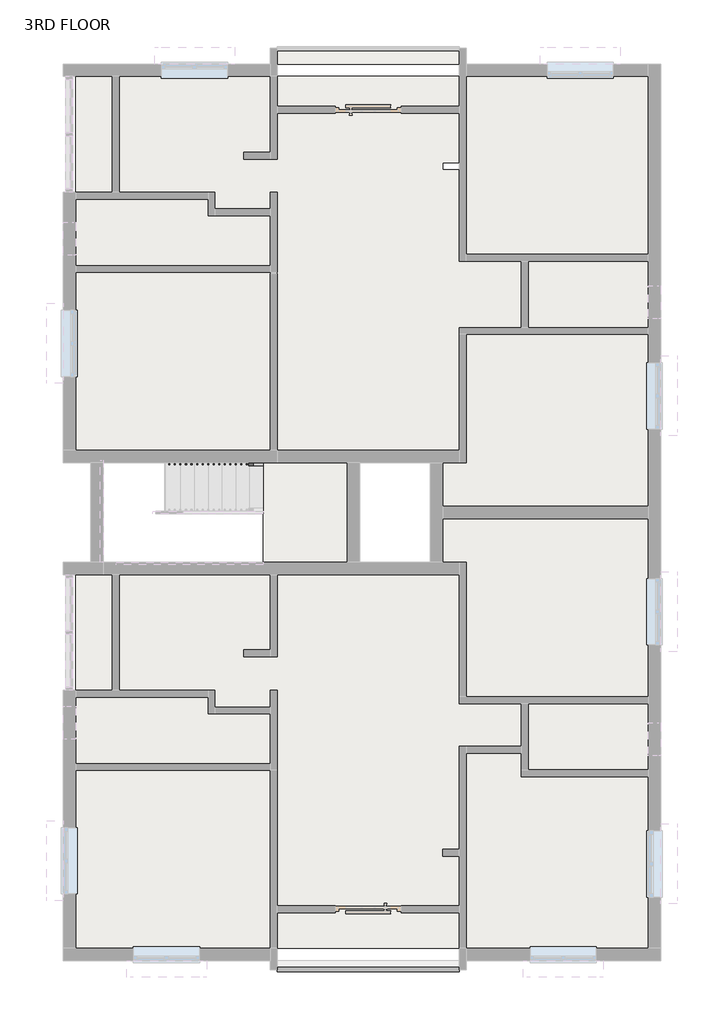
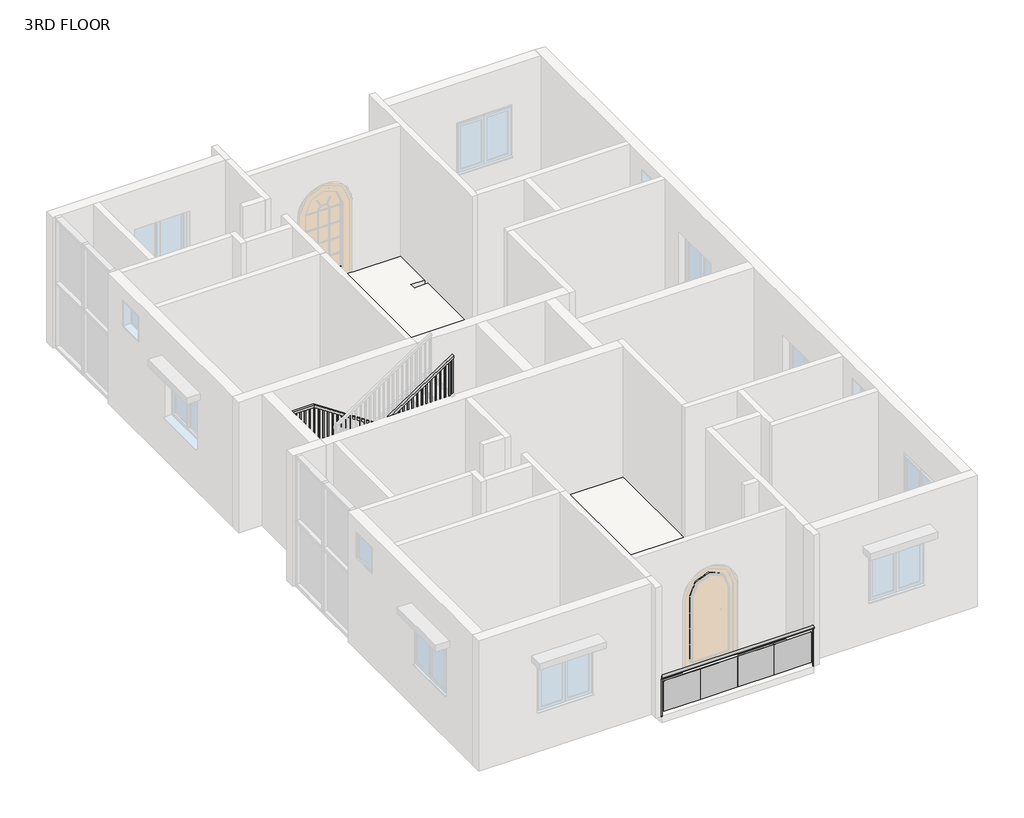
# One storey, part 3 of 4: 5 slabs, 2 railings.
"""IFC4 building model written with IfcOpenShell, lengths in millimetres."""

from ifc_helpers import new_model, si_unit, point, frame, origin, place, context, project, spatial, polyline, ellipse_curve, trimmed, outline, extrude, faceted_brep, element, save
from ifc_brep_helpers import plane_surface, extruded_surface, advanced_brep

model = new_model("IFC4")

# Units and contexts
model_context = context("Model", 3, world=origin())
ifc_project = project(units=[si_unit("LENGTHUNIT", "METRE", prefix="MILLI")], contexts=[model_context])

# Site, building, storey
site = spatial("IfcSite", under=ifc_project)
building = spatial("IfcBuilding", under=site)
storey = spatial("IfcBuildingStorey", under=building, Name="3RD FLOOR", Elevation=12192.0)

# Railings
placement = place(None, origin())
element("IfcRailing", 1, ObjectType="Glass Panel - Bottom Fill 2", at=placement, inside=storey, context=model_context, shape_type="SolidModel", body=[
    advanced_brep(
    [(-2494.0012202, -3358.1292559, 13106.4), (-2494.0012202, -3434.3292559, 13106.4), (858.7987798, -3358.1292559, 13106.4), (858.7987798, -3434.3292559, 13106.4)],
    [
        (0, 1, ellipse_curve(frame((-2494.0012202, -3396.2292559, 13106.4), z_axis=(-1.0, 0.0, 0.0), x_axis=(0.0, -1.0, 0.0)), 38.1, 28.575)),
        (1, 0, ellipse_curve(frame((-2494.0012202, -3396.2292559, 13106.4), z_axis=(-1.0, 0.0, 0.0), x_axis=(0.0, -1.0, 0.0)), 38.1, 28.575)),
        (2, 3, ellipse_curve(frame((858.7987798, -3396.2292559, 13106.4), z_axis=(1.0, 0.0, 0.0), x_axis=(0.0, -1.0, 0.0)), 38.1, 28.575)),
        (3, 2, ellipse_curve(frame((858.7987798, -3396.2292559, 13106.4), z_axis=(1.0, 0.0, 0.0), x_axis=(0.0, -1.0, 0.0)), 38.1, 28.575)),
        (0, 2),
        (3, 1),
    ],
    [
        plane_surface(frame((-2494.0012202, -3396.2292559, 13106.4), z_axis=(-1.0, 0.0, 0.0), x_axis=(0.0, 1.0, 0.0))),
        plane_surface(frame((858.7987798, -3396.2292559, 13106.4), z_axis=(1.0, 0.0, 0.0), x_axis=(0.0, 1.0, 0.0))),
        extruded_surface(trimmed(ellipse_curve(frame((858.7987798, -3396.2292559, 13106.4), z_axis=(-1.0, 0.0, 0.0), x_axis=(0.0, -1.0, 0.0)), 38.1, 28.575), [point((858.7987798, -3358.1292559, 13106.4))], [point((858.7987798, -3434.3292559, 13106.4))], True, "CARTESIAN"), (-3352.7999999999997, 0.0, 0.0), 3352.7999999999997),
        extruded_surface(trimmed(ellipse_curve(frame((858.7987798, -3396.2292559, 13106.4), z_axis=(-1.0, 0.0, 0.0), x_axis=(0.0, -1.0, 0.0)), 38.1, 28.575), [point((858.7987798, -3434.3292559, 13106.4))], [point((858.7987798, -3358.1292559, 13106.4))], True, "CARTESIAN"), (-3352.7999999999997, 0.0, 0.0), 3352.7999999999997),
    ],
    [
        (0, [[1, 2]]),
        (1, [[3, 4]]),
        (2, [[-1, 5, -4, 6]]),
        (3, [[-2, -6, -3, -5]]),
    ],
),
    extrude(outline(polyline([(-4.8012202, -3402.7644129), (-4.8012202, -3396.4144129), (807.9987798, -3396.4144129), (807.9987798, -3402.7644129), (-4.8012202, -3402.7644129)])), frame((0.0, 0.0, 12293.6), z_axis=(0.0, 0.0, 1.0), x_axis=(1.0, 0.0, 0.0)), (0.0, 0.0, 1.0), 711.2),
    extrude(outline(polyline([(-817.6012202, -3402.7644129), (-817.6012202, -3396.4144129), (-4.8012202, -3396.4144129), (-4.8012202, -3402.7644129), (-817.6012202, -3402.7644129)])), frame((0.0, 0.0, 12293.6), z_axis=(0.0, 0.0, 1.0), x_axis=(1.0, 0.0, 0.0)), (0.0, 0.0, 1.0), 711.2),
    extrude(outline(polyline([(-1630.4012202, -3402.7644129), (-1630.4012202, -3396.4144129), (-817.6012202, -3396.4144129), (-817.6012202, -3402.7644129), (-1630.4012202, -3402.7644129)])), frame((0.0, 0.0, 12293.6), z_axis=(0.0, 0.0, 1.0), x_axis=(1.0, 0.0, 0.0)), (0.0, 0.0, 1.0), 711.2),
    extrude(outline(polyline([(-2443.2012202, -3402.7644129), (-2443.2012202, -3396.4144129), (-1630.4012202, -3396.4144129), (-1630.4012202, -3402.7644129), (-2443.2012202, -3402.7644129)])), frame((0.0, 0.0, 12293.6), z_axis=(0.0, 0.0, 1.0), x_axis=(1.0, 0.0, 0.0)), (0.0, 0.0, 1.0), 711.2),
    extrude(outline(polyline([(846.0987798, -3386.7042559), (865.1487798, -3386.7042559), (865.1487798, -3405.7542559), (846.0987798, -3405.7542559), (846.0987798, -3386.7042559)])), frame((0.0, 0.0, 12192.0), z_axis=(0.0, 0.0, 1.0), x_axis=(1.0, 0.0, 0.0)), (0.0, 0.0, 1.0), 885.825),
    extrude(outline(polyline([(-2500.3512202, -3386.7042559), (-2481.3012202, -3386.7042559), (-2481.3012202, -3405.7542559), (-2500.3512202, -3405.7542559), (-2500.3512202, -3386.7042559)])), frame((0.0, 0.0, 12192.0), z_axis=(0.0, 0.0, 1.0), x_axis=(1.0, 0.0, 0.0)), (0.0, 0.0, 1.0), 885.825),
])
element("IfcRailing", 2, ObjectType="Handrail - Rectangular", at=placement, inside=storey, context=model_context, shape_type="SolidModel", body=[
    faceted_brep([(-2748.0012202, 5879.8309003, 13275.7333333), (-2748.0012202, 5879.8309003, 13214.6793317), (-2748.0012202, 5930.6309003, 13214.6793317), (-2748.0012202, 5930.6309003, 13275.7333333), (-4780.0012202, 5879.8309003, 14630.4), (-4795.3822226, 5879.8309003, 14579.6), (-4795.3822226, 5930.6309003, 14579.6), (-4780.0012202, 5930.6309003, 14630.4), (-5643.6012202, 5879.8309003, 14630.4), (-5643.6012202, 5879.8309003, 14579.6), (-5694.4012202, 5930.6309003, 14579.6), (-5694.4012202, 5930.6309003, 14630.4), (-5643.6012202, 4152.6309003, 14630.4), (-5643.6012202, 4152.6309003, 14579.6), (-5694.4012202, 4101.8309003, 14579.6), (-5694.4012202, 4101.8309003, 14630.4), (-5034.0012202, 4152.6309003, 14630.4), (-5018.6202178, 4152.6309003, 14579.6), (-5018.6202178, 4101.8309003, 14579.6), (-5034.0012202, 4101.8309003, 14630.4), (-2748.0012202, 4152.6309003, 16154.4), (-2748.0012202, 4101.8309003, 16154.4), (-2748.0012202, 4101.8309003, 16093.3459984), (-2748.0012202, 4152.6309003, 16093.3459984)], [[[0, 1, 2, 3]], [[1, 0, 4, 5]], [[2, 1, 5, 6]], [[3, 2, 6, 7]], [[0, 3, 7, 4]], [[5, 4, 8, 9]], [[6, 5, 9, 10]], [[7, 6, 10, 11]], [[4, 7, 11, 8]], [[9, 8, 12, 13]], [[10, 9, 13, 14]], [[11, 10, 14, 15]], [[8, 11, 15, 12]], [[13, 12, 16, 17]], [[14, 13, 17, 18]], [[15, 14, 18, 19]], [[12, 15, 19, 16]], [[20, 21, 22, 23]], [[17, 16, 20, 23]], [[18, 17, 23, 22]], [[19, 18, 22, 21]], [[16, 19, 21, 20]]]),
    extrude(outline(polyline([(16048.8959984, -2814.6762202), (16036.1959984, -2833.7262202), (15070.6666667, -2833.7262202), (15070.6666667, -2814.6762202), (16048.8959984, -2814.6762202)])), frame((0.0, 4117.7059003, 0.0), z_axis=(0.0, 1.0, 0.0), x_axis=(0.0, 0.0, 1.0)), (0.0, 0.0, 1.0), 19.05),
    extrude(outline(polyline([(15981.1626651, -2916.2762202), (15968.4626651, -2935.3262202), (15070.6666667, -2935.3262202), (15070.6666667, -2916.2762202), (15981.1626651, -2916.2762202)])), frame((0.0, 4117.7059003, 0.0), z_axis=(0.0, 1.0, 0.0), x_axis=(0.0, 0.0, 1.0)), (0.0, 0.0, 1.0), 19.05),
    extrude(outline(polyline([(15913.4293317, -3017.8762202), (15900.7293317, -3036.9262202), (14901.3333333, -3036.9262202), (14901.3333333, -3017.8762202), (15913.4293317, -3017.8762202)])), frame((0.0, 4117.7059003, 0.0), z_axis=(0.0, 1.0, 0.0), x_axis=(0.0, 0.0, 1.0)), (0.0, 0.0, 1.0), 19.05),
    extrude(outline(polyline([(15845.6959984, -3119.4762202), (15832.9959984, -3138.5262202), (14901.3333333, -3138.5262202), (14901.3333333, -3119.4762202), (15845.6959984, -3119.4762202)])), frame((0.0, 4117.7059003, 0.0), z_axis=(0.0, 1.0, 0.0), x_axis=(0.0, 0.0, 1.0)), (0.0, 0.0, 1.0), 19.05),
    extrude(outline(polyline([(15777.9626651, -3221.0762202), (15765.2626651, -3240.1262202), (14901.3333333, -3240.1262202), (14901.3333333, -3221.0762202), (15777.9626651, -3221.0762202)])), frame((0.0, 4117.7059003, 0.0), z_axis=(0.0, 1.0, 0.0), x_axis=(0.0, 0.0, 1.0)), (0.0, 0.0, 1.0), 19.05),
    extrude(outline(polyline([(15710.2293317, -3322.6762202), (15697.5293317, -3341.7262202), (14732.0, -3341.7262202), (14732.0, -3322.6762202), (15710.2293317, -3322.6762202)])), frame((0.0, 4117.7059003, 0.0), z_axis=(0.0, 1.0, 0.0), x_axis=(0.0, 0.0, 1.0)), (0.0, 0.0, 1.0), 19.05),
    extrude(outline(polyline([(15642.4959984, -3424.2762202), (15629.7959984, -3443.3262202), (14732.0, -3443.3262202), (14732.0, -3424.2762202), (15642.4959984, -3424.2762202)])), frame((0.0, 4117.7059003, 0.0), z_axis=(0.0, 1.0, 0.0), x_axis=(0.0, 0.0, 1.0)), (0.0, 0.0, 1.0), 19.05),
    extrude(outline(polyline([(15574.7626651, -3525.8762202), (15562.0626651, -3544.9262202), (14562.6666667, -3544.9262202), (14562.6666667, -3525.8762202), (15574.7626651, -3525.8762202)])), frame((0.0, 4117.7059003, 0.0), z_axis=(0.0, 1.0, 0.0), x_axis=(0.0, 0.0, 1.0)), (0.0, 0.0, 1.0), 19.05),
    extrude(outline(polyline([(15507.0293317, -3627.4762202), (15494.3293317, -3646.5262202), (14562.6666667, -3646.5262202), (14562.6666667, -3627.4762202), (15507.0293317, -3627.4762202)])), frame((0.0, 4117.7059003, 0.0), z_axis=(0.0, 1.0, 0.0), x_axis=(0.0, 0.0, 1.0)), (0.0, 0.0, 1.0), 19.05),
    extrude(outline(polyline([(15439.2959984, -3729.0762202), (15426.5959984, -3748.1262202), (14562.6666667, -3748.1262202), (14562.6666667, -3729.0762202), (15439.2959984, -3729.0762202)])), frame((0.0, 4117.7059003, 0.0), z_axis=(0.0, 1.0, 0.0), x_axis=(0.0, 0.0, 1.0)), (0.0, 0.0, 1.0), 19.05),
    extrude(outline(polyline([(15371.5626651, -3830.6762202), (15358.8626651, -3849.7262202), (14393.3333333, -3849.7262202), (14393.3333333, -3830.6762202), (15371.5626651, -3830.6762202)])), frame((0.0, 4117.7059003, 0.0), z_axis=(0.0, 1.0, 0.0), x_axis=(0.0, 0.0, 1.0)), (0.0, 0.0, 1.0), 19.05),
    extrude(outline(polyline([(15303.8293317, -3932.2762202), (15291.1293317, -3951.3262202), (14393.3333333, -3951.3262202), (14393.3333333, -3932.2762202), (15303.8293317, -3932.2762202)])), frame((0.0, 4117.7059003, 0.0), z_axis=(0.0, 1.0, 0.0), x_axis=(0.0, 0.0, 1.0)), (0.0, 0.0, 1.0), 19.05),
    extrude(outline(polyline([(15236.0959984, -4033.8762202), (15223.3959984, -4052.9262202), (14224.0, -4052.9262202), (14224.0, -4033.8762202), (15236.0959984, -4033.8762202)])), frame((0.0, 4117.7059003, 0.0), z_axis=(0.0, 1.0, 0.0), x_axis=(0.0, 0.0, 1.0)), (0.0, 0.0, 1.0), 19.05),
    extrude(outline(polyline([(15168.3626651, -4135.4762202), (15155.6626651, -4154.5262202), (14224.0, -4154.5262202), (14224.0, -4135.4762202), (15168.3626651, -4135.4762202)])), frame((0.0, 4117.7059003, 0.0), z_axis=(0.0, 1.0, 0.0), x_axis=(0.0, 0.0, 1.0)), (0.0, 0.0, 1.0), 19.05),
    extrude(outline(polyline([(15100.6293317, -4237.0762202), (15087.9293317, -4256.1262202), (14224.0, -4256.1262202), (14224.0, -4237.0762202), (15100.6293317, -4237.0762202)])), frame((0.0, 4117.7059003, 0.0), z_axis=(0.0, 1.0, 0.0), x_axis=(0.0, 0.0, 1.0)), (0.0, 0.0, 1.0), 19.05),
    extrude(outline(polyline([(15032.8959984, -4338.6762202), (15020.1959984, -4357.7262202), (14054.6666667, -4357.7262202), (14054.6666667, -4338.6762202), (15032.8959984, -4338.6762202)])), frame((0.0, 4117.7059003, 0.0), z_axis=(0.0, 1.0, 0.0), x_axis=(0.0, 0.0, 1.0)), (0.0, 0.0, 1.0), 19.05),
    extrude(outline(polyline([(14965.1626651, -4440.2762202), (14952.4626651, -4459.3262202), (14054.6666667, -4459.3262202), (14054.6666667, -4440.2762202), (14965.1626651, -4440.2762202)])), frame((0.0, 4117.7059003, 0.0), z_axis=(0.0, 1.0, 0.0), x_axis=(0.0, 0.0, 1.0)), (0.0, 0.0, 1.0), 19.05),
    extrude(outline(polyline([(14897.4293317, -4541.8762202), (14884.7293317, -4560.9262202), (13885.3333333, -4560.9262202), (13885.3333333, -4541.8762202), (14897.4293317, -4541.8762202)])), frame((0.0, 4117.7059003, 0.0), z_axis=(0.0, 1.0, 0.0), x_axis=(0.0, 0.0, 1.0)), (0.0, 0.0, 1.0), 19.05),
    extrude(outline(polyline([(14829.6959984, -4643.4762202), (14816.9959984, -4662.5262202), (13885.3333333, -4662.5262202), (13885.3333333, -4643.4762202), (14829.6959984, -4643.4762202)])), frame((0.0, 4117.7059003, 0.0), z_axis=(0.0, 1.0, 0.0), x_axis=(0.0, 0.0, 1.0)), (0.0, 0.0, 1.0), 19.05),
    extrude(outline(polyline([(14761.9626651, -4745.0762202), (14749.2626651, -4764.1262202), (13885.3333333, -4764.1262202), (13885.3333333, -4745.0762202), (14761.9626651, -4745.0762202)])), frame((0.0, 4117.7059003, 0.0), z_axis=(0.0, 1.0, 0.0), x_axis=(0.0, 0.0, 1.0)), (0.0, 0.0, 1.0), 19.05),
    extrude(outline(polyline([(14694.2293317, -4846.6762202), (14681.5293317, -4865.7262202), (13716.0, -4865.7262202), (13716.0, -4846.6762202), (14694.2293317, -4846.6762202)])), frame((0.0, 4117.7059003, 0.0), z_axis=(0.0, 1.0, 0.0), x_axis=(0.0, 0.0, 1.0)), (0.0, 0.0, 1.0), 19.05),
    extrude(outline(polyline([(14626.4959984, -4948.2762202), (14613.7959984, -4967.3262202), (13716.0, -4967.3262202), (13716.0, -4948.2762202), (14626.4959984, -4948.2762202)])), frame((0.0, 4117.7059003, 0.0), z_axis=(0.0, 1.0, 0.0), x_axis=(0.0, 0.0, 1.0)), (0.0, 0.0, 1.0), 19.05),
    extrude(outline(polyline([(-5068.9262202, 4117.7059003), (-5068.9262202, 4136.7559003), (-5049.8762202, 4136.7559003), (-5049.8762202, 4117.7059003), (-5068.9262202, 4117.7059003)])), frame((0.0, 0.0, 13716.0), z_axis=(0.0, 0.0, 1.0), x_axis=(1.0, 0.0, 0.0)), (0.0, 0.0, 1.0), 863.6),
    extrude(outline(polyline([(-5170.5262202, 4117.7059003), (-5170.5262202, 4136.7559003), (-5151.4762202, 4136.7559003), (-5151.4762202, 4117.7059003), (-5170.5262202, 4117.7059003)])), frame((0.0, 0.0, 13716.0), z_axis=(0.0, 0.0, 1.0), x_axis=(1.0, 0.0, 0.0)), (0.0, 0.0, 1.0), 863.6),
    extrude(outline(polyline([(-5272.1262202, 4117.7059003), (-5272.1262202, 4136.7559003), (-5253.0762202, 4136.7559003), (-5253.0762202, 4117.7059003), (-5272.1262202, 4117.7059003)])), frame((0.0, 0.0, 13716.0), z_axis=(0.0, 0.0, 1.0), x_axis=(1.0, 0.0, 0.0)), (0.0, 0.0, 1.0), 863.6),
    extrude(outline(polyline([(-5373.7262202, 4117.7059003), (-5373.7262202, 4136.7559003), (-5354.6762202, 4136.7559003), (-5354.6762202, 4117.7059003), (-5373.7262202, 4117.7059003)])), frame((0.0, 0.0, 13716.0), z_axis=(0.0, 0.0, 1.0), x_axis=(1.0, 0.0, 0.0)), (0.0, 0.0, 1.0), 863.6),
    extrude(outline(polyline([(-5475.3262202, 4117.7059003), (-5475.3262202, 4136.7559003), (-5456.2762202, 4136.7559003), (-5456.2762202, 4117.7059003), (-5475.3262202, 4117.7059003)])), frame((0.0, 0.0, 13716.0), z_axis=(0.0, 0.0, 1.0), x_axis=(1.0, 0.0, 0.0)), (0.0, 0.0, 1.0), 863.6),
    extrude(outline(polyline([(-5576.9262202, 4117.7059003), (-5576.9262202, 4136.7559003), (-5557.8762202, 4136.7559003), (-5557.8762202, 4117.7059003), (-5576.9262202, 4117.7059003)])), frame((0.0, 0.0, 13716.0), z_axis=(0.0, 0.0, 1.0), x_axis=(1.0, 0.0, 0.0)), (0.0, 0.0, 1.0), 863.6),
    extrude(outline(polyline([(-5678.5262202, 4187.5559003), (-5659.4762202, 4187.5559003), (-5659.4762202, 4168.5059003), (-5678.5262202, 4168.5059003), (-5678.5262202, 4187.5559003)])), frame((0.0, 0.0, 13716.0), z_axis=(0.0, 0.0, 1.0), x_axis=(1.0, 0.0, 0.0)), (0.0, 0.0, 1.0), 863.6),
    extrude(outline(polyline([(-5678.5262202, 4289.1559003), (-5659.4762202, 4289.1559003), (-5659.4762202, 4270.1059003), (-5678.5262202, 4270.1059003), (-5678.5262202, 4289.1559003)])), frame((0.0, 0.0, 13716.0), z_axis=(0.0, 0.0, 1.0), x_axis=(1.0, 0.0, 0.0)), (0.0, 0.0, 1.0), 863.6),
    extrude(outline(polyline([(-5678.5262202, 4390.7559003), (-5659.4762202, 4390.7559003), (-5659.4762202, 4371.7059003), (-5678.5262202, 4371.7059003), (-5678.5262202, 4390.7559003)])), frame((0.0, 0.0, 13716.0), z_axis=(0.0, 0.0, 1.0), x_axis=(1.0, 0.0, 0.0)), (0.0, 0.0, 1.0), 863.6),
    extrude(outline(polyline([(-5678.5262202, 4492.3559003), (-5659.4762202, 4492.3559003), (-5659.4762202, 4473.3059003), (-5678.5262202, 4473.3059003), (-5678.5262202, 4492.3559003)])), frame((0.0, 0.0, 13716.0), z_axis=(0.0, 0.0, 1.0), x_axis=(1.0, 0.0, 0.0)), (0.0, 0.0, 1.0), 863.6),
    extrude(outline(polyline([(-5678.5262202, 4593.9559003), (-5659.4762202, 4593.9559003), (-5659.4762202, 4574.9059003), (-5678.5262202, 4574.9059003), (-5678.5262202, 4593.9559003)])), frame((0.0, 0.0, 13716.0), z_axis=(0.0, 0.0, 1.0), x_axis=(1.0, 0.0, 0.0)), (0.0, 0.0, 1.0), 863.6),
    extrude(outline(polyline([(-5678.5262202, 4695.5559003), (-5659.4762202, 4695.5559003), (-5659.4762202, 4676.5059003), (-5678.5262202, 4676.5059003), (-5678.5262202, 4695.5559003)])), frame((0.0, 0.0, 13716.0), z_axis=(0.0, 0.0, 1.0), x_axis=(1.0, 0.0, 0.0)), (0.0, 0.0, 1.0), 863.6),
    extrude(outline(polyline([(-5678.5262202, 4797.1559003), (-5659.4762202, 4797.1559003), (-5659.4762202, 4778.1059003), (-5678.5262202, 4778.1059003), (-5678.5262202, 4797.1559003)])), frame((0.0, 0.0, 13716.0), z_axis=(0.0, 0.0, 1.0), x_axis=(1.0, 0.0, 0.0)), (0.0, 0.0, 1.0), 863.6),
    extrude(outline(polyline([(-5678.5262202, 4898.7559003), (-5659.4762202, 4898.7559003), (-5659.4762202, 4879.7059003), (-5678.5262202, 4879.7059003), (-5678.5262202, 4898.7559003)])), frame((0.0, 0.0, 13716.0), z_axis=(0.0, 0.0, 1.0), x_axis=(1.0, 0.0, 0.0)), (0.0, 0.0, 1.0), 863.6),
    extrude(outline(polyline([(-5678.5262202, 5000.3559003), (-5659.4762202, 5000.3559003), (-5659.4762202, 4981.3059003), (-5678.5262202, 4981.3059003), (-5678.5262202, 5000.3559003)])), frame((0.0, 0.0, 13716.0), z_axis=(0.0, 0.0, 1.0), x_axis=(1.0, 0.0, 0.0)), (0.0, 0.0, 1.0), 863.6),
    extrude(outline(polyline([(-5678.5262202, 5101.9559003), (-5659.4762202, 5101.9559003), (-5659.4762202, 5082.9059003), (-5678.5262202, 5082.9059003), (-5678.5262202, 5101.9559003)])), frame((0.0, 0.0, 13716.0), z_axis=(0.0, 0.0, 1.0), x_axis=(1.0, 0.0, 0.0)), (0.0, 0.0, 1.0), 863.6),
    extrude(outline(polyline([(-5678.5262202, 5203.5559003), (-5659.4762202, 5203.5559003), (-5659.4762202, 5184.5059003), (-5678.5262202, 5184.5059003), (-5678.5262202, 5203.5559003)])), frame((0.0, 0.0, 13716.0), z_axis=(0.0, 0.0, 1.0), x_axis=(1.0, 0.0, 0.0)), (0.0, 0.0, 1.0), 863.6),
    extrude(outline(polyline([(-5678.5262202, 5305.1559003), (-5659.4762202, 5305.1559003), (-5659.4762202, 5286.1059003), (-5678.5262202, 5286.1059003), (-5678.5262202, 5305.1559003)])), frame((0.0, 0.0, 13716.0), z_axis=(0.0, 0.0, 1.0), x_axis=(1.0, 0.0, 0.0)), (0.0, 0.0, 1.0), 863.6),
    extrude(outline(polyline([(-5678.5262202, 5406.7559003), (-5659.4762202, 5406.7559003), (-5659.4762202, 5387.7059003), (-5678.5262202, 5387.7059003), (-5678.5262202, 5406.7559003)])), frame((0.0, 0.0, 13716.0), z_axis=(0.0, 0.0, 1.0), x_axis=(1.0, 0.0, 0.0)), (0.0, 0.0, 1.0), 863.6),
    extrude(outline(polyline([(-5678.5262202, 5508.3559003), (-5659.4762202, 5508.3559003), (-5659.4762202, 5489.3059003), (-5678.5262202, 5489.3059003), (-5678.5262202, 5508.3559003)])), frame((0.0, 0.0, 13716.0), z_axis=(0.0, 0.0, 1.0), x_axis=(1.0, 0.0, 0.0)), (0.0, 0.0, 1.0), 863.6),
    extrude(outline(polyline([(-5678.5262202, 5609.9559003), (-5659.4762202, 5609.9559003), (-5659.4762202, 5590.9059003), (-5678.5262202, 5590.9059003), (-5678.5262202, 5609.9559003)])), frame((0.0, 0.0, 13716.0), z_axis=(0.0, 0.0, 1.0), x_axis=(1.0, 0.0, 0.0)), (0.0, 0.0, 1.0), 863.6),
    extrude(outline(polyline([(-5678.5262202, 5711.5559003), (-5659.4762202, 5711.5559003), (-5659.4762202, 5692.5059003), (-5678.5262202, 5692.5059003), (-5678.5262202, 5711.5559003)])), frame((0.0, 0.0, 13716.0), z_axis=(0.0, 0.0, 1.0), x_axis=(1.0, 0.0, 0.0)), (0.0, 0.0, 1.0), 863.6),
    extrude(outline(polyline([(-5678.5262202, 5813.1559003), (-5659.4762202, 5813.1559003), (-5659.4762202, 5794.1059003), (-5678.5262202, 5794.1059003), (-5678.5262202, 5813.1559003)])), frame((0.0, 0.0, 13716.0), z_axis=(0.0, 0.0, 1.0), x_axis=(1.0, 0.0, 0.0)), (0.0, 0.0, 1.0), 863.6),
    extrude(outline(polyline([(-5583.2762202, 5914.7559003), (-5583.2762202, 5895.7059003), (-5602.3262202, 5895.7059003), (-5602.3262202, 5914.7559003), (-5583.2762202, 5914.7559003)])), frame((0.0, 0.0, 13716.0), z_axis=(0.0, 0.0, 1.0), x_axis=(1.0, 0.0, 0.0)), (0.0, 0.0, 1.0), 863.6),
    extrude(outline(polyline([(-5481.6762202, 5914.7559003), (-5481.6762202, 5895.7059003), (-5500.7262202, 5895.7059003), (-5500.7262202, 5914.7559003), (-5481.6762202, 5914.7559003)])), frame((0.0, 0.0, 13716.0), z_axis=(0.0, 0.0, 1.0), x_axis=(1.0, 0.0, 0.0)), (0.0, 0.0, 1.0), 863.6),
    extrude(outline(polyline([(-5380.0762202, 5914.7559003), (-5380.0762202, 5895.7059003), (-5399.1262202, 5895.7059003), (-5399.1262202, 5914.7559003), (-5380.0762202, 5914.7559003)])), frame((0.0, 0.0, 13716.0), z_axis=(0.0, 0.0, 1.0), x_axis=(1.0, 0.0, 0.0)), (0.0, 0.0, 1.0), 863.6),
    extrude(outline(polyline([(-5278.4762202, 5914.7559003), (-5278.4762202, 5895.7059003), (-5297.5262202, 5895.7059003), (-5297.5262202, 5914.7559003), (-5278.4762202, 5914.7559003)])), frame((0.0, 0.0, 13716.0), z_axis=(0.0, 0.0, 1.0), x_axis=(1.0, 0.0, 0.0)), (0.0, 0.0, 1.0), 863.6),
    extrude(outline(polyline([(-5176.8762202, 5914.7559003), (-5176.8762202, 5895.7059003), (-5195.9262202, 5895.7059003), (-5195.9262202, 5914.7559003), (-5176.8762202, 5914.7559003)])), frame((0.0, 0.0, 13716.0), z_axis=(0.0, 0.0, 1.0), x_axis=(1.0, 0.0, 0.0)), (0.0, 0.0, 1.0), 863.6),
    extrude(outline(polyline([(-5075.2762202, 5914.7559003), (-5075.2762202, 5895.7059003), (-5094.3262202, 5895.7059003), (-5094.3262202, 5914.7559003), (-5075.2762202, 5914.7559003)])), frame((0.0, 0.0, 13716.0), z_axis=(0.0, 0.0, 1.0), x_axis=(1.0, 0.0, 0.0)), (0.0, 0.0, 1.0), 863.6),
    extrude(outline(polyline([(-4973.6762202, 5914.7559003), (-4973.6762202, 5895.7059003), (-4992.7262202, 5895.7059003), (-4992.7262202, 5914.7559003), (-4973.6762202, 5914.7559003)])), frame((0.0, 0.0, 13716.0), z_axis=(0.0, 0.0, 1.0), x_axis=(1.0, 0.0, 0.0)), (0.0, 0.0, 1.0), 863.6),
    extrude(outline(polyline([(-4872.0762202, 5914.7559003), (-4872.0762202, 5895.7059003), (-4891.1262202, 5895.7059003), (-4891.1262202, 5914.7559003), (-4872.0762202, 5914.7559003)])), frame((0.0, 0.0, 13716.0), z_axis=(0.0, 0.0, 1.0), x_axis=(1.0, 0.0, 0.0)), (0.0, 0.0, 1.0), 863.6),
    extrude(outline(polyline([(14562.9959984, -4770.4762202), (14575.6959984, -4789.5262202), (13716.0, -4789.5262202), (13716.0, -4770.4762202), (14562.9959984, -4770.4762202)])), frame((0.0, 5895.7059003, 0.0), z_axis=(0.0, 1.0, 0.0), x_axis=(0.0, 0.0, 1.0)), (0.0, 0.0, 1.0), 19.05),
    extrude(outline(polyline([(14495.2626651, -4668.8762202), (14507.9626651, -4687.9262202), (13546.6666667, -4687.9262202), (13546.6666667, -4668.8762202), (14495.2626651, -4668.8762202)])), frame((0.0, 5895.7059003, 0.0), z_axis=(0.0, 1.0, 0.0), x_axis=(0.0, 0.0, 1.0)), (0.0, 0.0, 1.0), 19.05),
    extrude(outline(polyline([(14427.5293317, -4567.2762202), (14440.2293317, -4586.3262202), (13546.6666667, -4586.3262202), (13546.6666667, -4567.2762202), (14427.5293317, -4567.2762202)])), frame((0.0, 5895.7059003, 0.0), z_axis=(0.0, 1.0, 0.0), x_axis=(0.0, 0.0, 1.0)), (0.0, 0.0, 1.0), 19.05),
    extrude(outline(polyline([(14359.7959984, -4465.6762202), (14372.4959984, -4484.7262202), (13377.3333333, -4484.7262202), (13377.3333333, -4465.6762202), (14359.7959984, -4465.6762202)])), frame((0.0, 5895.7059003, 0.0), z_axis=(0.0, 1.0, 0.0), x_axis=(0.0, 0.0, 1.0)), (0.0, 0.0, 1.0), 19.05),
    extrude(outline(polyline([(14292.0626651, -4364.0762202), (14304.7626651, -4383.1262202), (13377.3333333, -4383.1262202), (13377.3333333, -4364.0762202), (14292.0626651, -4364.0762202)])), frame((0.0, 5895.7059003, 0.0), z_axis=(0.0, 1.0, 0.0), x_axis=(0.0, 0.0, 1.0)), (0.0, 0.0, 1.0), 19.05),
    extrude(outline(polyline([(14224.3293317, -4262.4762202), (14237.0293317, -4281.5262202), (13377.3333333, -4281.5262202), (13377.3333333, -4262.4762202), (14224.3293317, -4262.4762202)])), frame((0.0, 5895.7059003, 0.0), z_axis=(0.0, 1.0, 0.0), x_axis=(0.0, 0.0, 1.0)), (0.0, 0.0, 1.0), 19.05),
    extrude(outline(polyline([(14156.5959984, -4160.8762202), (14169.2959984, -4179.9262202), (13208.0, -4179.9262202), (13208.0, -4160.8762202), (14156.5959984, -4160.8762202)])), frame((0.0, 5895.7059003, 0.0), z_axis=(0.0, 1.0, 0.0), x_axis=(0.0, 0.0, 1.0)), (0.0, 0.0, 1.0), 19.05),
    extrude(outline(polyline([(14088.8626651, -4059.2762202), (14101.5626651, -4078.3262202), (13208.0, -4078.3262202), (13208.0, -4059.2762202), (14088.8626651, -4059.2762202)])), frame((0.0, 5895.7059003, 0.0), z_axis=(0.0, 1.0, 0.0), x_axis=(0.0, 0.0, 1.0)), (0.0, 0.0, 1.0), 19.05),
    extrude(outline(polyline([(14021.1293317, -3957.6762202), (14033.8293317, -3976.7262202), (13038.6666667, -3976.7262202), (13038.6666667, -3957.6762202), (14021.1293317, -3957.6762202)])), frame((0.0, 5895.7059003, 0.0), z_axis=(0.0, 1.0, 0.0), x_axis=(0.0, 0.0, 1.0)), (0.0, 0.0, 1.0), 19.05),
    extrude(outline(polyline([(13953.3959984, -3856.0762202), (13966.0959984, -3875.1262202), (13038.6666667, -3875.1262202), (13038.6666667, -3856.0762202), (13953.3959984, -3856.0762202)])), frame((0.0, 5895.7059003, 0.0), z_axis=(0.0, 1.0, 0.0), x_axis=(0.0, 0.0, 1.0)), (0.0, 0.0, 1.0), 19.05),
    extrude(outline(polyline([(13885.6626651, -3754.4762202), (13898.3626651, -3773.5262202), (13038.6666667, -3773.5262202), (13038.6666667, -3754.4762202), (13885.6626651, -3754.4762202)])), frame((0.0, 5895.7059003, 0.0), z_axis=(0.0, 1.0, 0.0), x_axis=(0.0, 0.0, 1.0)), (0.0, 0.0, 1.0), 19.05),
    extrude(outline(polyline([(13817.9293317, -3652.8762202), (13830.6293317, -3671.9262202), (12869.3333333, -3671.9262202), (12869.3333333, -3652.8762202), (13817.9293317, -3652.8762202)])), frame((0.0, 5895.7059003, 0.0), z_axis=(0.0, 1.0, 0.0), x_axis=(0.0, 0.0, 1.0)), (0.0, 0.0, 1.0), 19.05),
    extrude(outline(polyline([(13750.1959984, -3551.2762202), (13762.8959984, -3570.3262202), (12869.3333333, -3570.3262202), (12869.3333333, -3551.2762202), (13750.1959984, -3551.2762202)])), frame((0.0, 5895.7059003, 0.0), z_axis=(0.0, 1.0, 0.0), x_axis=(0.0, 0.0, 1.0)), (0.0, 0.0, 1.0), 19.05),
    extrude(outline(polyline([(13682.4626651, -3449.6762202), (13695.1626651, -3468.7262202), (12700.0, -3468.7262202), (12700.0, -3449.6762202), (13682.4626651, -3449.6762202)])), frame((0.0, 5895.7059003, 0.0), z_axis=(0.0, 1.0, 0.0), x_axis=(0.0, 0.0, 1.0)), (0.0, 0.0, 1.0), 19.05),
    extrude(outline(polyline([(13614.7293317, -3348.0762202), (13627.4293317, -3367.1262202), (12700.0, -3367.1262202), (12700.0, -3348.0762202), (13614.7293317, -3348.0762202)])), frame((0.0, 5895.7059003, 0.0), z_axis=(0.0, 1.0, 0.0), x_axis=(0.0, 0.0, 1.0)), (0.0, 0.0, 1.0), 19.05),
    extrude(outline(polyline([(13546.9959984, -3246.4762202), (13559.6959984, -3265.5262202), (12700.0, -3265.5262202), (12700.0, -3246.4762202), (13546.9959984, -3246.4762202)])), frame((0.0, 5895.7059003, 0.0), z_axis=(0.0, 1.0, 0.0), x_axis=(0.0, 0.0, 1.0)), (0.0, 0.0, 1.0), 19.05),
    extrude(outline(polyline([(13479.2626651, -3144.8762202), (13491.9626651, -3163.9262202), (12530.6666667, -3163.9262202), (12530.6666667, -3144.8762202), (13479.2626651, -3144.8762202)])), frame((0.0, 5895.7059003, 0.0), z_axis=(0.0, 1.0, 0.0), x_axis=(0.0, 0.0, 1.0)), (0.0, 0.0, 1.0), 19.05),
    extrude(outline(polyline([(13411.5293317, -3043.2762202), (13424.2293317, -3062.3262202), (12530.6666667, -3062.3262202), (12530.6666667, -3043.2762202), (13411.5293317, -3043.2762202)])), frame((0.0, 5895.7059003, 0.0), z_axis=(0.0, 1.0, 0.0), x_axis=(0.0, 0.0, 1.0)), (0.0, 0.0, 1.0), 19.05),
    extrude(outline(polyline([(13343.7959984, -2941.6762202), (13356.4959984, -2960.7262202), (12361.3333333, -2960.7262202), (12361.3333333, -2941.6762202), (13343.7959984, -2941.6762202)])), frame((0.0, 5895.7059003, 0.0), z_axis=(0.0, 1.0, 0.0), x_axis=(0.0, 0.0, 1.0)), (0.0, 0.0, 1.0), 19.05),
    extrude(outline(polyline([(13276.0626651, -2840.0762202), (13288.7626651, -2859.1262202), (12361.3333333, -2859.1262202), (12361.3333333, -2840.0762202), (13276.0626651, -2840.0762202)])), frame((0.0, 5895.7059003, 0.0), z_axis=(0.0, 1.0, 0.0), x_axis=(0.0, 0.0, 1.0)), (0.0, 0.0, 1.0), 19.05),
    extrude(outline(polyline([(-5678.5262202, 4136.7559003), (-5659.4762202, 4136.7559003), (-5659.4762202, 4117.7059003), (-5678.5262202, 4117.7059003), (-5678.5262202, 4136.7559003)])), frame((0.0, 0.0, 13716.0), z_axis=(0.0, 0.0, 1.0), x_axis=(1.0, 0.0, 0.0)), (0.0, 0.0, 1.0), 863.6),
    extrude(outline(polyline([(-5659.4762202, 5914.7559003), (-5659.4762202, 5895.7059003), (-5678.5262202, 5895.7059003), (-5678.5262202, 5914.7559003), (-5659.4762202, 5914.7559003)])), frame((0.0, 0.0, 13716.0), z_axis=(0.0, 0.0, 1.0), x_axis=(1.0, 0.0, 0.0)), (0.0, 0.0, 1.0), 863.6),
    extrude(outline(polyline([(16093.3459984, -2748.0012202), (16080.6459984, -2767.0512202), (15070.6666667, -2767.0512202), (15070.6666667, -2748.0012202), (16093.3459984, -2748.0012202)])), frame((0.0, 4117.7059003, 0.0), z_axis=(0.0, 1.0, 0.0), x_axis=(0.0, 0.0, 1.0)), (0.0, 0.0, 1.0), 19.05),
    extrude(outline(polyline([(13214.6793317, -2748.0012202), (13227.3793317, -2767.0512202), (12361.3333333, -2767.0512202), (12361.3333333, -2748.0012202), (13214.6793317, -2748.0012202)])), frame((0.0, 5895.7059003, 0.0), z_axis=(0.0, 1.0, 0.0), x_axis=(0.0, 0.0, 1.0)), (0.0, 0.0, 1.0), 19.05),
])

# Slabs
element("IfcSlab", 3, ObjectType="FLOORING 6\"", at=placement, inside=storey, context=model_context, shape_type="SweptSolid", body=[
    extrude(outline(polyline([(-2621.0012202, 11645.6309003), (-3103.6012202, 11645.6309003), (-3103.6012202, 11518.6309003), (-2557.5012202, 11518.6309003), (-2494.0012202, 11518.6309003), (-2494.0012202, 13042.6309003), (858.7987798, 13042.6309003), (858.7987798, 11455.1309003), (553.9987798, 11455.1309003), (553.9987798, 11328.1309003), (858.7987798, 11328.1309003), (858.7987798, 9639.0309003), (2001.7987798, 9639.0309003), (2001.7987798, 8419.8309003), (858.7987798, 8419.8309003), (858.7987798, 6159.2309003), (-2494.0012202, 6159.2309003), (-2494.0012202, 9435.8309003), (-2494.0012202, 10909.0309003), (-2621.0012202, 10909.0309003), (-2621.0012202, 10604.2309003), (-3637.0012202, 10604.2309003), (-3637.0012202, 10909.0309003), (-6202.4012202, 10909.0309003), (-6202.4012202, 13042.6309003), (-2621.0012202, 13042.6309003), (-2621.0012202, 11645.6309003)])), frame((0.0, 0.0, 12039.6), z_axis=(0.0, 0.0, 1.0), x_axis=(1.0, 0.0, 0.0)), (0.0, 0.0, 1.0), 152.4),
])
element("IfcSlab", 4, ObjectType="FLOORING 6\"", at=placement, inside=storey, context=model_context, shape_type="SweptSolid", body=[
    extrude(outline(polyline([(4338.5987798, 13042.6309003), (4338.5987798, 9766.0309003), (985.7987798, 9766.0309003), (985.7987798, 13042.6309003), (4338.5987798, 13042.6309003)])), frame((0.0, 0.0, 12039.6), z_axis=(0.0, 0.0, 1.0), x_axis=(1.0, 0.0, 0.0)), (0.0, 0.0, 1.0), 152.4),
    extrude(outline(polyline([(4338.5987798, 9639.0309003), (4338.5987798, 8419.8309003), (2128.7987798, 8419.8309003), (2128.7987798, 9639.0309003), (4338.5987798, 9639.0309003)])), frame((0.0, 0.0, 12039.6), z_axis=(0.0, 0.0, 1.0), x_axis=(1.0, 0.0, 0.0)), (0.0, 0.0, 1.0), 152.4),
    extrude(outline(polyline([(-2621.0012202, 9435.8309003), (-2621.0012202, 6159.2309003), (-6202.4012202, 6159.2309003), (-6202.4012202, 9435.8309003), (-2621.0012202, 9435.8309003)])), frame((0.0, 0.0, 12039.6), z_axis=(0.0, 0.0, 1.0), x_axis=(1.0, 0.0, 0.0)), (0.0, 0.0, 1.0), 152.4),
    extrude(outline(polyline([(-2621.0012202, 9562.8309003), (-6202.4012202, 9562.8309003), (-6202.4012202, 10782.0309003), (-3764.0012202, 10782.0309003), (-3764.0012202, 10477.2309003), (-2621.0012202, 10477.2309003), (-2621.0012202, 9562.8309003)])), frame((0.0, 0.0, 12039.6), z_axis=(0.0, 0.0, 1.0), x_axis=(1.0, 0.0, 0.0)), (0.0, 0.0, 1.0), 152.4),
    extrude(outline(polyline([(553.9987798, 5930.6309003), (985.7987798, 5930.6309003), (985.7987798, 8292.8309003), (4338.5987798, 8292.8309003), (4338.5987798, 5130.5309003), (553.9987798, 5130.5309003), (553.9987798, 5930.6309003)])), frame((0.0, 0.0, 12039.6), z_axis=(0.0, 0.0, 1.0), x_axis=(1.0, 0.0, 0.0)), (0.0, 0.0, 1.0), 152.4),
])
element("IfcSlab", 5, ObjectType="FLOORING 6\"", at=placement, inside=storey, context=model_context, shape_type="SweptSolid", body=[
    extrude(outline(polyline([(985.7987798, 583.9309003), (2001.7987798, 583.9309003), (2001.7987798, 152.1309003), (4338.5987798, 152.1309003), (4338.5987798, -3010.1690997), (985.7987798, -3010.1690997), (985.7987798, 583.9309003)])), frame((0.0, 0.0, 12039.6), z_axis=(0.0, 0.0, 1.0), x_axis=(1.0, 0.0, 0.0)), (0.0, 0.0, 1.0), 152.4),
    extrude(outline(polyline([(-6203.9887202, -3010.1690997), (-6203.9887202, 266.4309003), (-2621.0012202, 266.4309003), (-2621.0012202, -3010.1690997), (-6203.9887202, -3010.1690997)])), frame((0.0, 0.0, 12039.6), z_axis=(0.0, 0.0, 1.0), x_axis=(1.0, 0.0, 0.0)), (0.0, 0.0, 1.0), 152.4),
    extrude(outline(polyline([(-2621.0012202, 393.4309003), (-6203.9887202, 393.4309003), (-6203.9887202, 1612.6309003), (-3764.0012202, 1612.6309003), (-3764.0012202, 1307.8309003), (-2621.0012202, 1307.8309003), (-2621.0012202, 393.4309003)])), frame((0.0, 0.0, 12039.6), z_axis=(0.0, 0.0, 1.0), x_axis=(1.0, 0.0, 0.0)), (0.0, 0.0, 1.0), 152.4),
    extrude(outline(polyline([(858.7987798, -3010.1690997), (-2494.0012202, -3010.1690997), (-2494.0012202, 1739.6309003), (-2621.0012202, 1739.6309003), (-2621.0012202, 1434.8309003), (-3637.0012202, 1434.8309003), (-3637.0012202, 1739.6309003), (-6203.9887202, 1739.6309003), (-6203.9887202, 3873.2309003), (-2621.0012202, 3873.2309003), (-2621.0012202, 2488.9309003), (-3103.6012202, 2488.9309003), (-3103.6012202, 2361.9309003), (-2494.0012202, 2361.9309003), (-2494.0012202, 3873.2309003), (858.7987798, 3873.2309003), (858.7987798, 1498.3309003), (2001.7987798, 1498.3309003), (2001.7987798, 710.9309003), (858.7987798, 710.9309003), (858.7987798, -3010.1690997)])), frame((0.0, 0.0, 12039.6), z_axis=(0.0, 0.0, 1.0), x_axis=(1.0, 0.0, 0.0)), (0.0, 0.0, 1.0), 152.4),
    extrude(outline(polyline([(985.7987798, 1625.3309003), (985.7987798, 4101.8309003), (553.9987798, 4101.8309003), (553.9987798, 4901.9309003), (4338.5987798, 4901.9309003), (4338.5987798, 1625.3309003), (985.7987798, 1625.3309003)])), frame((0.0, 0.0, 12039.6), z_axis=(0.0, 0.0, 1.0), x_axis=(1.0, 0.0, 0.0)), (0.0, 0.0, 1.0), 152.4),
    extrude(outline(polyline([(-2748.0012202, 4000.2309003), (-2748.0012202, 5981.4309003), (-2748.0012202, 6032.2309003), (-2494.0012202, 6032.2309003), (-2494.0012202, 5930.6309003), (-1198.6012202, 5930.6309003), (-1198.6012202, 4101.8309003), (-2494.0012202, 4101.8309003), (-2494.0012202, 4000.2309003), (-2748.0012202, 4000.2309003)])), frame((0.0, 0.0, 12039.6), z_axis=(0.0, 0.0, 1.0), x_axis=(1.0, 0.0, 0.0)), (0.0, 0.0, 1.0), 152.4),
])
element("IfcSlab", 6, ObjectType="bathroom tiles", at=placement, inside=storey, context=model_context, shape_type="SweptSolid", body=[
    extrude(outline(polyline([(858.7987798, 13563.3309003), (858.7987798, 13271.2309003), (-2494.0012202, 13271.2309003), (-2494.0012202, 13563.3309003), (858.7987798, 13563.3309003)])), frame((0.0, 0.0, 12039.6), z_axis=(0.0, 0.0, 1.0), x_axis=(1.0, 0.0, 0.0)), (0.0, 0.0, 1.0), 152.4),
])
element("IfcSlab", 7, ObjectType="bathroom tiles", at=placement, inside=storey, context=model_context, shape_type="SweptSolid", body=[
    extrude(outline(polyline([(4338.5987798, 1498.3309003), (4338.5987798, 279.1309003), (2128.7987798, 279.1309003), (2128.7987798, 1498.3309003), (4338.5987798, 1498.3309003)])), frame((0.0, 0.0, 12039.6), z_axis=(0.0, 0.0, 1.0), x_axis=(1.0, 0.0, 0.0)), (0.0, 0.0, 1.0), 152.4),
])

save(model, "model.ifc")

# Revit data of these elements
# Type "Glass Panel - Bottom Fill 2"
#   Assembly Code = "C2010400"
#   built-in parameter 1008612 = 0.0416667 (stored number, unit not read)
#   built-in parameter 1008611 = 0.0416667 (stored number, unit not read)
#   built-in parameter 1008609 = 0.333333 (stored number, unit not read)
#   built-in parameter 1008604 = 0.166667 (stored number, unit not read)
#   built-in parameter 1008603 = 0.166667 (stored number, unit not read)
#   Railing Height = 3' - 0"
#   built-in parameter 1008630 = 2
#   built-in parameter 1008610 = 2
#   built-in parameter 1008618 = Baluster - Square : 3/4"
# Type "Handrail - Rectangular"
#   Assembly Code = "C2010400"
#   built-in parameter 1008612 = 0.0416667 (stored number, unit not read)
#   built-in parameter 1008611 = 0.0416667 (stored number, unit not read)
#   built-in parameter 1008609 = 0.333333 (stored number, unit not read)
#   built-in parameter 1008604 = 0.166667 (stored number, unit not read)
#   built-in parameter 1008603 = 0.166667 (stored number, unit not read)
#   Railing Height = 3' - 0"
#   built-in parameter 1008630 = 2
#   built-in parameter 1008610 = 2
#   built-in parameter 1008618 = Baluster - Square : 3/4"
# Type "FLOORING 6\""
#   Assembly Code = "B1010"
#   Function = 0
#   Layers, outside or top first: 0' - 6" "MARBLE FLOORING" (function 1)
# Type "bathroom tiles"
#   Assembly Code = "B1010"
#   Function = 0
#   Layers, outside or top first: 0' - 6" "tile flooring" (function 1)
# Element 1 (IfcRailing, "Glass Panel - Bottom Fill 2")
#   Phase Created = New Construction
#   Materials on its faces: "Glass"
# Element 2 (IfcRailing, "Handrail - Rectangular")
#   Phase Created = New Construction
# Element 3 (IfcSlab, "FLOORING 6\"")
#   built-in parameter 1001955 = -1.5708 (stored number, unit not read)
#   Height Offset From Level = 0' - 0"
#   Phase Created = New Construction
#   Materials on its faces: "MARBLE FLOORING"
# Element 4 (IfcSlab, "FLOORING 6\"")
#   Height Offset From Level = 0' - 0"
#   Phase Created = New Construction
#   Materials on its faces: "MARBLE FLOORING"
# Element 5 (IfcSlab, "FLOORING 6\"")
#   built-in parameter 1001955 = 1.5708 (stored number, unit not read)
#   Height Offset From Level = 0' - 0"
#   Phase Created = New Construction
#   Materials on its faces: "MARBLE FLOORING"
# Elements 6, 7 (IfcSlab, "bathroom tiles")
#   Height Offset From Level = 0' - 0"
#   Phase Created = New Construction
#   Materials on its faces: "tile flooring"
# Materials
#   "MARBLE FLOORING": class "Generic", colour RGB 120 120 120, transparency 0, Cost = 0
#   "tile flooring": class "Generic", colour RGB 120 120 120, transparency 0, Cost = 0
#   "Glass": class "Glass", colour RGB 0 128 192, transparency 0.75, Description = "Soda Lime Glass", Cost = 0
